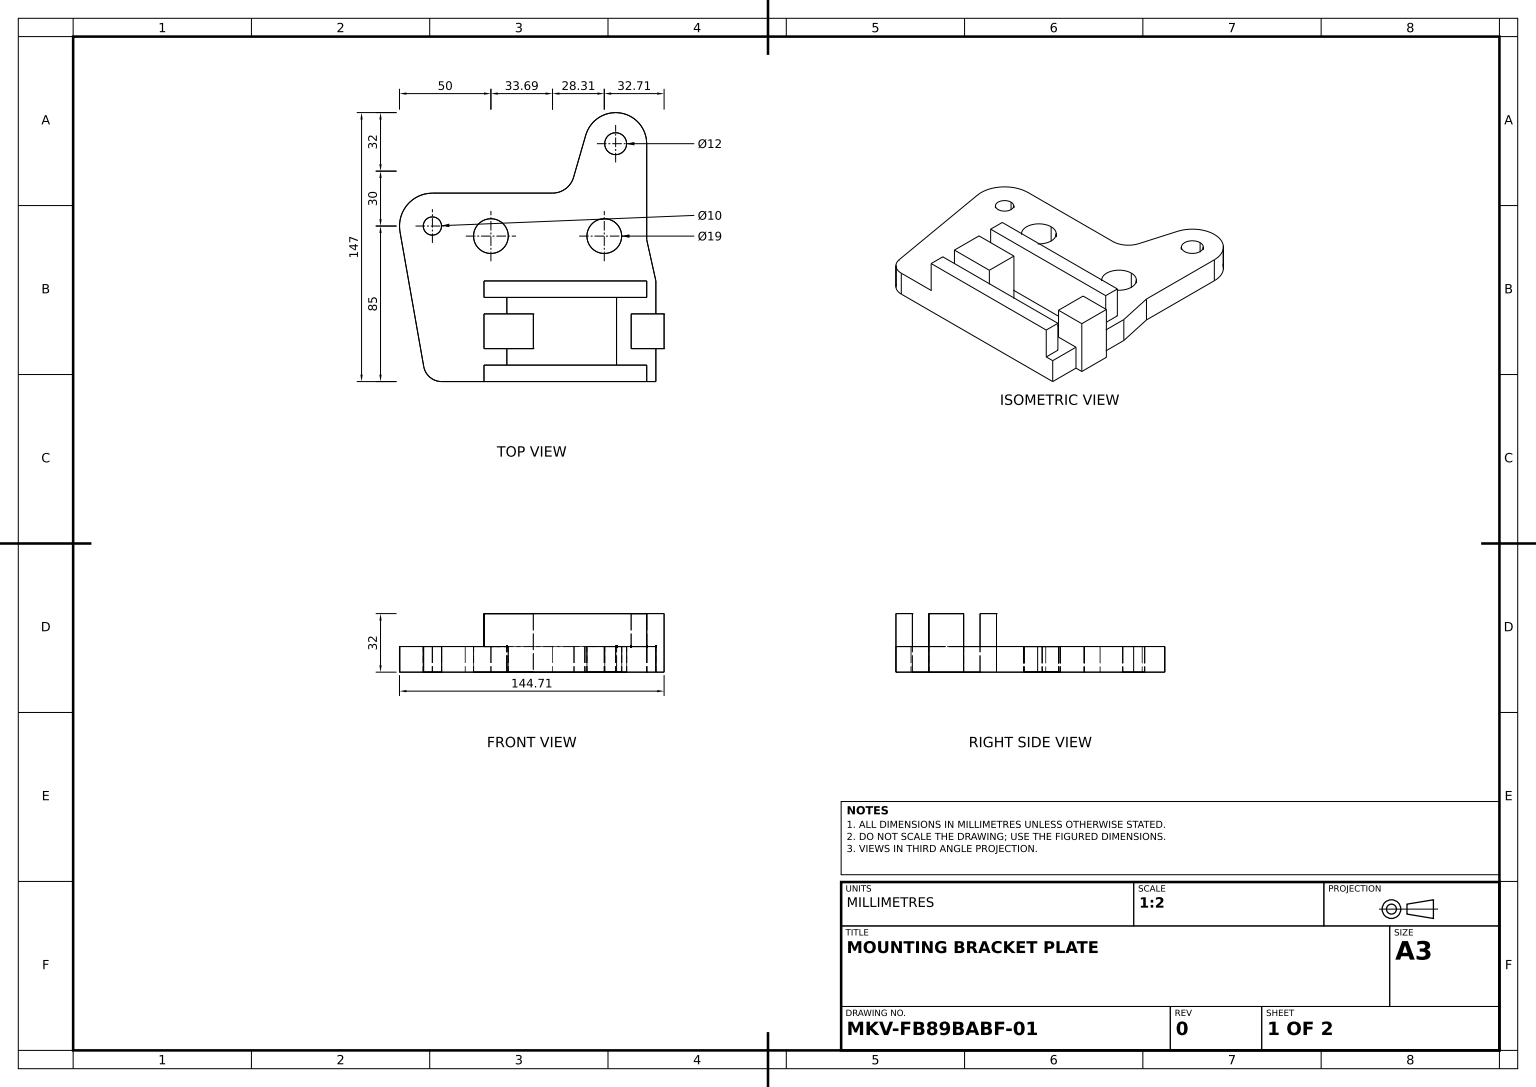
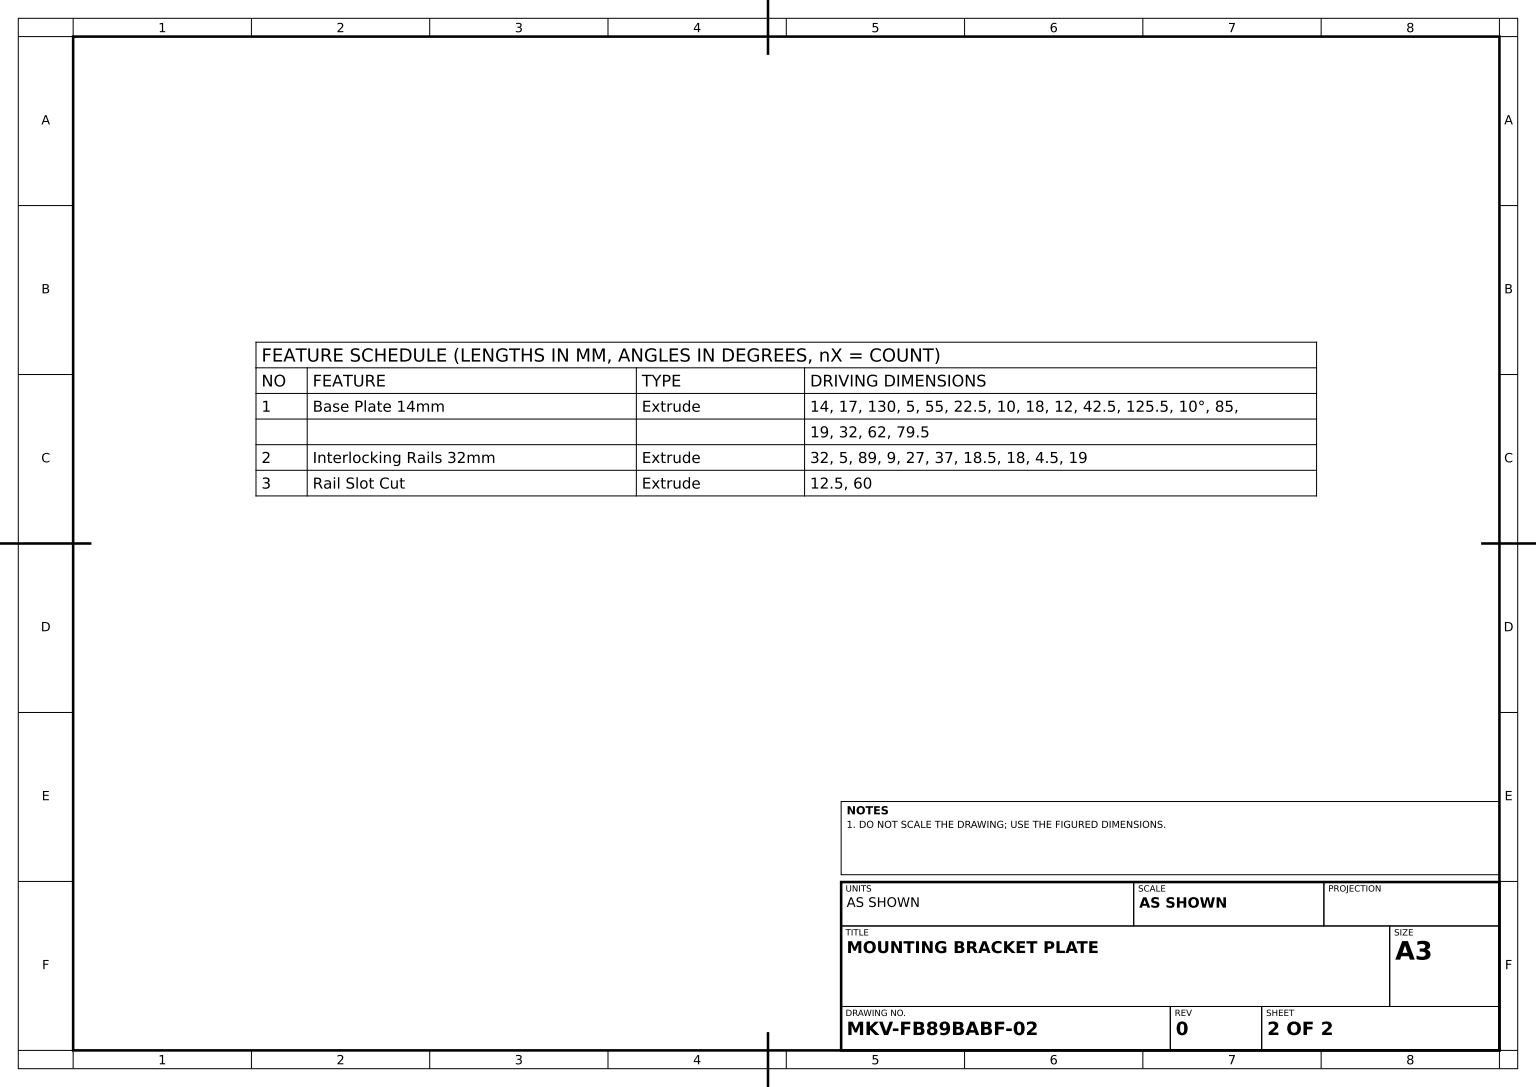
SolidWorks part; units mm, degrees
material "Plain Carbon Steel"
ref_plane "Front Plane" through (0, 0, 0) normal (0, 0, 1) x (1, 0, 0)
ref_plane "Top Plane" through (0, 0, 0) normal (0, 1, 0) x (1, 0, 0)
ref_plane "Right Plane" through (0, 0, 0) normal (1, 0, 0) x (0, 0, -1)
sketch "Base Plate Profile Sketch" plane through (0, 0, 0) normal (0, 1, 0) x (1, 0, 0)
  line L0 (0, 0) -> (-117.109, 0)
  line L1 (-126.9571, 8.2635) -> (-139.9367, 81.8743)
  line L2 (-122.2101, 103) -> (-56.5227, 103)
  line L3 (-44.9946, 111.6679) -> (-38.3315, 134.7205)
  line L4 (0, 0) -> (0, 55)
  line L5 (0, 55) -> (-5, 77.5)
  line L6 (-5, 77.5) -> (-5, 130)
  line L7 (-44.9946, 111.6679) -> (-49.8758, 94.7803) construction
  line L8 (-56.5227, 103) -> (-13.7205, 103) construction
  line L9 (-126.9571, 8.2635) -> (-124.0429, -8.2635) construction
  line L10 (-117.109, 0) -> (-149.9163, 0) construction
  line L11 (-125.5, 0) -> (-125.5, 19.5557) construction
  arc A0 (-5, 130) -> (-38.3315, 134.7205) centre (-22, 130) ccw
  arc A1 (-117.109, 0) -> (-126.9571, 8.2635) centre (-117.109, 10) cw
  arc A2 (-139.9367, 81.8743) -> (-122.2101, 103) centre (-122.2101, 85) cw
  arc A3 (-56.5227, 103) -> (-44.9946, 111.6679) centre (-56.5227, 115) ccw
  circle A4 centre (-22, 130) radius 6
  circle A5 centre (-122.2101, 85) radius 5
  circle A6 centre (-90.2101, 79.5) radius 9.5
  circle A7 centre (-28.2101, 79.5) radius 9.5
  point P7 (-47.5, 103)
  point P12 (-125.5, 0)
  dimension "D1" = 17
  dimension "D6" = 10
  dimension "D7" = 18
  dimension "D8" = 12
  dimension "D10" = 12
  dimension "D14" = 10
  dimension "D15" = 19
  dimension "D17" = 19
  dimension "D2" = 130
  dimension "D3" = 5
  dimension "D4" = 55
  dimension "D5" = 22.5
  dimension "D9" = 42.5
  dimension "D11" = 125.5
  dimension "D12" = 10
  dimension "D13" = 85
  dimension "D16" = 32
  dimension "D18" = 62
  dimension "D19" = 79.5
extrude "Base Plate 14mm" add sketch "Base Plate Profile Sketch" along normal blind 14
sketch "Interlocking Rails Sketch" plane through (0, 0, 0) normal (0, 1, 0) x (1, 0, 0)
  line L0 (-117.109, 0) -> (0, 0) construction
  line L1 (-94, 0) -> (-5, 0)
  line L2 (-94, 0) -> (-94, 9)
  line L3 (-94, 9) -> (-5, 9)
  line L4 (-5, 0) -> (-5, 9)
  line L6 (-94, 18) -> (-67, 18)
  line L7 (-94, 18) -> (-94, 37)
  line L8 (-94, 37) -> (-67, 37)
  line L9 (-67, 18) -> (-67, 37)
  line L10 (-94, 46) -> (-5, 46)
  line L11 (-94, 46) -> (-94, 55)
  line L12 (-94, 55) -> (-5, 55)
  line L13 (-5, 46) -> (-5, 55)
  line L14 (-13.5, 37) -> (4.5, 37)
  line L15 (-13.5, 37) -> (-13.5, 18)
  line L16 (-13.5, 18) -> (4.5, 18)
  line L17 (4.5, 37) -> (4.5, 18)
  point P11 (-94, 27.5)
  dimension "D1" = 5
  dimension "D2" = 89
  dimension "D3" = 9
  dimension "D4" = 27
  dimension "D5" = 18.5
  dimension "D6" = 9
  dimension "D7" = 37
  dimension "D8" = 18
  dimension "D9" = 4.5
  dimension "D10" = 19
extrude "Interlocking Rails 32mm" add sketch "Interlocking Rails Sketch" along normal blind 32
sketch "Rail Slot Sketch" plane through (0, 14, 0) normal (0, 1, 0) x (1, 0, 0)
  line L0 (-81.5, 46) -> (-81.5, 37)
  line L1 (-5, 46) -> (-94, 46) construction
  line L2 (-94, 37) -> (-67, 37) construction
  line L3 (-81.5, 18) -> (-81.5, 9)
  line L4 (-67, 18) -> (-94, 18) construction
  line L5 (-5, 9) -> (-94, 9) construction
  line L6 (-94, 0) -> (-94, 9) construction
  line L7 (-67, 37) -> (-94, 37) construction
  line L8 (-67, 37) -> (-67, 18) construction
  line L9 (-94, 9) -> (-5, 9) construction
  line L10 (-94, 46) -> (-5, 46) construction
  line L11 (-67, 37) -> (-81.5, 37)
  line L12 (-67, 18) -> (-81.5, 18)
  line L13 (-67, 37) -> (-67, 18)
  line L14 (-81.5, 9) -> (-21.5, 9)
  line L15 (-81.5, 46) -> (-21.5, 46)
  line L16 (-21.5, 46) -> (-21.5, 9)
  dimension "D1" = 12.5
  dimension "D2" = 60
extrude "Rail Slot Cut" cut sketch "Rail Slot Sketch" against normal up to next
